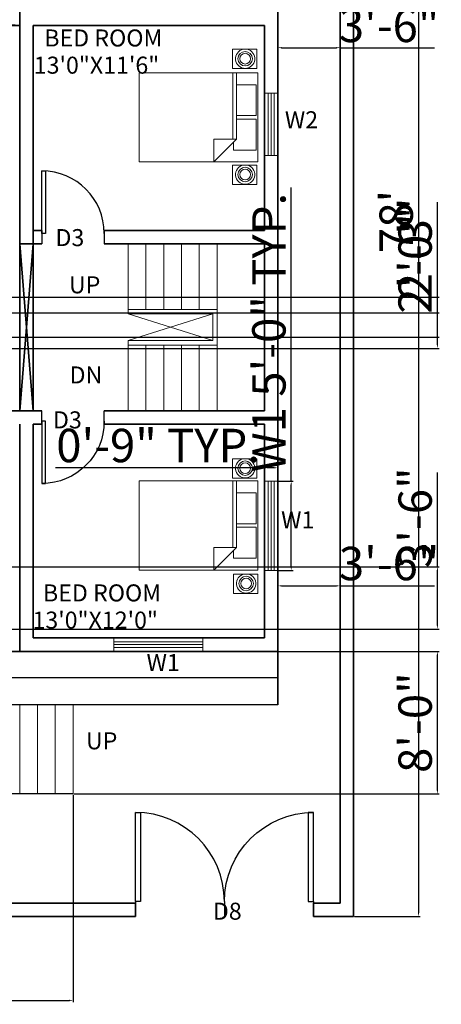
# Model space of a CAD drawing. Units: inches. Extents: x 164 to 1038, y 98 to 1358.
# Tile 3 of 4: x 754 to 1038, y 151 to 814. Entities that reach past the tile are written whole.
import ezdxf

# ---------------------------------------------------------------- set-up
doc = ezdxf.new("R2010")
doc.units = ezdxf.units.IN
for name, color, linetype, lineweight in [('A-ANNO-DIMS', 7, 'Continuous', 18), ('A-ANNO-TEXT', 3, 'Continuous', 18), ('A-AREA-IDEN', 3, 'Continuous', 18), ('A-FLOR', 7, 'Continuous', 25), ('C-SITE-GATE', 6, 'Continuous', 25), ('C-SITE-WALL', 7, 'Continuous', 35), ('door', 6, 'Continuous', 25), ('furniture', 2, 'Continuous', 18), ('staircase', 4, 'Continuous', 18), ('wall', 7, 'Continuous', 35), ('window', 10, 'Continuous', 18)]:
    doc.layers.add(name, color=color, linetype=linetype, lineweight=lineweight)
doc.styles.get("Standard").update_dxf_attribs({"font": 'arial.ttf'})
doc.dimstyles.new('ISO-25', dxfattribs={"dimtxt": 22.5, "dimasz": 2.5, "dimexe": 1.25, "dimexo": 0.625, "dimtad": 1, "dimdec": 0, "dimlunit": 3, "dimtxsty": 'Standard', "dimcen": 2.5, "dimadec": 0, "dimazin": 0, "dimtfac": 1, "dimtdec": 0, "dimtmove": 0, "dimatfit": 3, "dimfxl": 1, "dimarcsym": 0})

# ---------------------------------------------------------------- blocks, each defined once
blk = doc.blocks.new('*U3')
for p, q in [((0, 0), (0, -5)), ((30, 0), (30, -5))]:
    blk.add_line(p, q)
blk.add_lwpolyline([(0, 0), (0, 30), (1.75, 30), (1.75, 0)], close=True)
blk.add_arc((0, 0), 30, 0, 90)
blk = doc.blocks.new('Bed - Queen')
for p, q in [((0, -80.00003), (0, 0)), ((0, 0), (59.99999, 0)), ((59.99999, 0), (59.99999, -80.00003)), ((7.99999, -1.2), (28.79998, -1.2)), ((7.99999, -14.4), (7.99999, -1.2)), ((28.79998, -1.2), (28.79998, -14.4)), ((31.19999, -1.2), (51.99999, -1.2)), ((31.19999, -14.4), (31.19999, -1.2)), ((51.99999, -1.2), (51.99999, -16.4)), ((0, -14.4), (44.8, -14.4)), ((44.8, -16.8), (0, -16.8)), ((59.99999, -29.6), (44.8, -14.4)), ((44.8, -14.4), (44.8, -29.6)), ((51.99999, -16.4), (46.79936, -16.4)), ((44.8, -29.6), (59.99999, -29.6)), ((59.99999, -80.00003), (0, -80.00003))]:
    blk.add_line(p, q)
blk = doc.blocks.new('*D19')
at = {"layer": 'A-ANNO-DIMS', "color": 0, "lineweight": -2, "transparency": 16777216}
for p, q in [((979.69, 1145.87), (1024.11, 1145.87)), ((1022.86, 1143.37), (1022.86, 212.37)), ((979.69, 209.87), (1024.11, 209.87))]:
    blk.add_line(p, q, dxfattribs=at)
at = {"layer": 'A-ANNO-DIMS', "color": 0, "transparency": 16777216}
for points in [[(1022.44, 1143.37), (1023.28, 1143.37), (1022.86, 1145.87)], [(1022.44, 212.37), (1023.28, 212.37), (1022.86, 209.87)]]:
    blk.add_solid(points, dxfattribs=at)
at = {"layer": 'Defpoints', "color": 0, "transparency": 16777216}
for p in [(979.07, 1145.87), (979.07, 209.87), (1022.86, 209.87)]:
    blk.add_point(p, dxfattribs=at)
at = {"layer": 'A-ANNO-DIMS', "color": 0, "transparency": 16777216, "insert": (1010.75, 677.87), "char_height": 22.5, "attachment_point": 5, "rotation": 90}
blk.add_mtext("78'", dxfattribs=at)
blk = doc.blocks.new('*D25')
at = {"layer": 'A-ANNO-DIMS', "color": 0, "lineweight": -2, "transparency": 16777216}
for p, q in [((928.07, 429.88), (928.07, 433.73)), ((930.57, 432.48), (967.57, 432.48)), ((970.07, 429.88), (970.07, 433.73)), ((970.07, 432.48), (1033.61, 432.48))]:
    blk.add_line(p, q, dxfattribs=at)
at = {"layer": 'A-ANNO-DIMS', "color": 0, "transparency": 16777216}
for points in [[(930.57, 432.9), (930.57, 432.07), (928.07, 432.48)], [(967.57, 432.9), (967.57, 432.07), (970.07, 432.48)]]:
    blk.add_solid(points, dxfattribs=at)
at = {"layer": 'Defpoints', "color": 0, "transparency": 16777216}
for p in [(970.07, 432.48), (928.07, 429.26), (970.07, 429.26)]:
    blk.add_point(p, dxfattribs=at)
at = {"layer": 'A-ANNO-DIMS', "color": 0, "transparency": 16777216, "insert": (1003.09, 444.6), "char_height": 22.5, "attachment_point": 5}
blk.add_mtext('3\'-6"', dxfattribs=at)
blk = doc.blocks.new('*D28')
at = {"layer": 'A-ANNO-DIMS', "color": 0, "lineweight": -2, "transparency": 16777216}
for p, q in [((928.07, 772.18), (928.07, 796.13)), ((970.07, 772.18), (970.07, 796.13)), ((930.57, 794.88), (967.57, 794.88)), ((970.07, 794.88), (1033.61, 794.88))]:
    blk.add_line(p, q, dxfattribs=at)
at = {"layer": 'A-ANNO-DIMS', "color": 0, "transparency": 16777216}
for points in [[(930.57, 795.3), (930.57, 794.46), (928.07, 794.88)], [(967.57, 795.3), (967.57, 794.46), (970.07, 794.88)]]:
    blk.add_solid(points, dxfattribs=at)
at = {"layer": 'Defpoints', "color": 0, "transparency": 16777216}
for p in [(970.07, 794.88), (928.07, 771.56), (970.07, 771.56)]:
    blk.add_point(p, dxfattribs=at)
at = {"layer": 'A-ANNO-DIMS', "color": 0, "transparency": 16777216, "insert": (1003.09, 807), "char_height": 22.5, "attachment_point": 5}
blk.add_mtext('3\'-6"', dxfattribs=at)
blk = doc.blocks.new('WINDOW-W1')
for p, q in [((0, 9), (0, 0)), ((60.11, 9), (60.11, 0)), ((0, 6.5), (60.11, 6.5)), ((0, 4.5), (60.11, 4.5)), ((0, 2.5), (60.11, 2.5))]:
    blk.add_line(p, q)
blk = doc.blocks.new('WINDOW-W2')
for p, q in [((0, 9), (0, 0)), ((42.02, 9), (42.02, 0)), ((0, 6.5), (42.02, 6.5)), ((0, 4.5), (42.02, 4.5)), ((0, 2.5), (42.02, 2.5))]:
    blk.add_line(p, q)
blk = doc.blocks.new('BEDSIDE-TABLE')
blk.add_lwpolyline([(0, 13.01), (16.36, 13.01), (16.36, 0), (0, 0)], close=True)
for radius in [4.87, 3.63]:
    blk.add_circle((8.46, 6.65), radius)
blk.add_arc((8.46, 6.65), 6.51, 102.02927, 77.97073)
blk.add_arc((8.46, 6.65), 6.51, 102.02927, 77.97073)
blk = doc.blocks.new('*D34')
at = {"layer": 'A-ANNO-DIMS', "color": 0, "lineweight": -2, "transparency": 16777216}
for p, q in [((937.08, 502.97), (937.08, 700.67)), ((928.69, 502.97), (938.33, 502.97)), ((937.08, 445.36), (937.08, 500.47)), ((928.69, 442.86), (938.33, 442.86))]:
    blk.add_line(p, q, dxfattribs=at)
at = {"layer": 'A-ANNO-DIMS', "color": 0, "transparency": 16777216}
for points in [[(936.67, 500.47), (937.5, 500.47), (937.08, 502.97)], [(936.67, 445.36), (937.5, 445.36), (937.08, 442.86)]]:
    blk.add_solid(points, dxfattribs=at)
at = {"layer": 'Defpoints', "color": 0, "transparency": 16777216}
for p in [(928.07, 502.97), (937.08, 502.97), (928.07, 442.86)]:
    blk.add_point(p, dxfattribs=at)
at = {"layer": 'A-ANNO-DIMS', "color": 0, "transparency": 16777216, "insert": (924.97, 603.07), "char_height": 22.5, "attachment_point": 5, "rotation": 90}
blk.add_mtext('W1 5\'-0" TYP.', dxfattribs=at)
blk = doc.blocks.new('*D35')
at = {"layer": 'A-ANNO-DIMS', "color": 0, "lineweight": -2, "transparency": 16777216}
for p, q in [((919.07, 511.99), (778.17, 511.99)), ((919.07, 503.6), (919.07, 513.24)), ((925.57, 511.99), (921.57, 511.99)), ((928.07, 503.6), (928.07, 513.24))]:
    blk.add_line(p, q, dxfattribs=at)
at = {"layer": 'A-ANNO-DIMS', "color": 0, "transparency": 16777216}
for points in [[(921.57, 512.4), (921.57, 511.57), (919.07, 511.99)], [(925.57, 512.4), (925.57, 511.57), (928.07, 511.99)]]:
    blk.add_solid(points, dxfattribs=at)
at = {"layer": 'Defpoints', "color": 0, "transparency": 16777216}
for p in [(919.07, 511.99), (919.07, 502.97), (928.07, 502.97)]:
    blk.add_point(p, dxfattribs=at)
at = {"layer": 'A-ANNO-DIMS', "color": 0, "transparency": 16777216, "insert": (847.37, 524.1), "char_height": 22.5, "attachment_point": 5}
blk.add_mtext('0\'-9" TYP.', dxfattribs=at)
blk = doc.blocks.new('*D56')
at = {"layer": 'A-ANNO-DIMS', "color": 0, "lineweight": -2, "transparency": 16777216}
for p, q in [((1035.62, 616.37), (1035.62, 680.31)), ((510.19, 616.37), (1036.87, 616.37)), ((1035.62, 594.87), (1035.62, 613.87)), ((510.19, 592.37), (1036.87, 592.37))]:
    blk.add_line(p, q, dxfattribs=at)
at = {"layer": 'A-ANNO-DIMS', "color": 0, "transparency": 16777216}
for points in [[(1035.2, 613.87), (1036.03, 613.87), (1035.62, 616.37)], [(1035.2, 594.87), (1036.03, 594.87), (1035.62, 592.37)]]:
    blk.add_solid(points, dxfattribs=at)
at = {"layer": 'Defpoints', "color": 0, "transparency": 16777216}
for p in [(509.57, 616.37), (1035.62, 616.37), (509.57, 592.37)]:
    blk.add_point(p, dxfattribs=at)
at = {"layer": 'A-ANNO-DIMS', "color": 0, "transparency": 16777216, "insert": (1023.5, 649.59), "char_height": 22.5, "attachment_point": 5, "rotation": 90}
blk.add_mtext('2\'-0"', dxfattribs=at)
blk = doc.blocks.new('*D58')
at = {"layer": 'A-ANNO-DIMS', "color": 0, "lineweight": -2, "transparency": 16777216}
for p, q in [((1035.62, 626.87), (1035.62, 690.81)), ((400.69, 626.87), (1036.87, 626.87)), ((1035.62, 602.37), (1035.62, 624.37)), ((400.69, 599.87), (1036.87, 599.87))]:
    blk.add_line(p, q, dxfattribs=at)
at = {"layer": 'A-ANNO-DIMS', "color": 0, "transparency": 16777216}
for points in [[(1035.2, 624.37), (1036.03, 624.37), (1035.62, 626.87)], [(1035.2, 602.37), (1036.03, 602.37), (1035.62, 599.87)]]:
    blk.add_solid(points, dxfattribs=at)
at = {"layer": 'Defpoints', "color": 0, "transparency": 16777216}
for p in [(400.07, 626.87), (1035.62, 626.87), (400.07, 599.87)]:
    blk.add_point(p, dxfattribs=at)
at = {"layer": 'A-ANNO-DIMS', "color": 0, "transparency": 16777216, "insert": (1023.5, 660.09), "char_height": 22.5, "attachment_point": 5, "rotation": 90}
blk.add_mtext('2\'-3"', dxfattribs=at)
blk = doc.blocks.new('*D59')
at = {"layer": 'A-ANNO-DIMS', "color": 0, "lineweight": -2, "transparency": 16777216}
for p, q in [((1035.62, 445.37), (1035.62, 508.91)), ((607.69, 445.37), (1036.87, 445.37)), ((1035.62, 405.87), (1035.62, 442.87)), ((607.69, 403.37), (1036.87, 403.37))]:
    blk.add_line(p, q, dxfattribs=at)
at = {"layer": 'A-ANNO-DIMS', "color": 0, "transparency": 16777216}
for points in [[(1035.2, 442.87), (1036.03, 442.87), (1035.62, 445.37)], [(1035.2, 405.87), (1036.03, 405.87), (1035.62, 403.37)]]:
    blk.add_solid(points, dxfattribs=at)
at = {"layer": 'Defpoints', "color": 0, "transparency": 16777216}
for p in [(607.07, 445.37), (1035.62, 445.37), (607.07, 403.37)]:
    blk.add_point(p, dxfattribs=at)
at = {"layer": 'A-ANNO-DIMS', "color": 0, "transparency": 16777216, "insert": (1023.5, 478.39), "char_height": 22.5, "attachment_point": 5, "rotation": 90}
blk.add_mtext('3\'-6"', dxfattribs=at)
blk = doc.blocks.new('*D60')
at = {"layer": 'A-ANNO-DIMS', "color": 0, "lineweight": -2, "transparency": 16777216}
for p, q in [((568.07, 291.74), (568.07, 152.07)), ((790.07, 291.74), (790.07, 152.07)), ((570.57, 153.32), (787.57, 153.32))]:
    blk.add_line(p, q, dxfattribs=at)
at = {"layer": 'A-ANNO-DIMS', "color": 0, "transparency": 16777216}
for points in [[(570.57, 153.73), (570.57, 152.9), (568.07, 153.32)], [(787.57, 153.73), (787.57, 152.9), (790.07, 153.32)]]:
    blk.add_solid(points, dxfattribs=at)
at = {"layer": 'Defpoints', "color": 0, "transparency": 16777216}
for p in [(568.07, 292.37), (790.07, 292.37), (790.07, 153.32)]:
    blk.add_point(p, dxfattribs=at)
at = {"layer": 'A-ANNO-DIMS', "color": 0, "transparency": 16777216, "insert": (679.07, 165.43), "char_height": 22.5, "attachment_point": 5}
blk.add_mtext('18\'-6"', dxfattribs=at)
blk = doc.blocks.new('*D61')
at = {"layer": 'A-ANNO-DIMS', "color": 0, "lineweight": -2, "transparency": 16777216}
for p, q in [((928.69, 388.37), (1036.87, 388.37)), ((1035.62, 294.87), (1035.62, 385.87)), ((790.69, 292.37), (1036.87, 292.37))]:
    blk.add_line(p, q, dxfattribs=at)
at = {"layer": 'A-ANNO-DIMS', "color": 0, "transparency": 16777216}
for points in [[(1035.2, 385.87), (1036.03, 385.87), (1035.62, 388.37)], [(1035.2, 294.87), (1036.03, 294.87), (1035.62, 292.37)]]:
    blk.add_solid(points, dxfattribs=at)
at = {"layer": 'Defpoints', "color": 0, "transparency": 16777216}
for p in [(928.07, 388.37), (1035.62, 388.37), (790.07, 292.37)]:
    blk.add_point(p, dxfattribs=at)
at = {"layer": 'A-ANNO-DIMS', "color": 0, "transparency": 16777216, "insert": (1023.5, 340.37), "char_height": 22.5, "attachment_point": 5, "rotation": 90}
blk.add_mtext('8\'-0"', dxfattribs=at)

msp = doc.modelspace()

# ---------------------------------------------------------------- linework, layer by layer
at = {"layer": 'A-FLOR'}
for p, q in [((715.07, 370.73), (928.07, 370.73)), ((928.07, 370.73), (928.07, 370.73)), ((928.07, 352.37), (715.07, 352.37)), ((790.07, 292.37), (568.07, 292.37))]:
    msp.add_line(p, q, dxfattribs=at)
at = {"layer": 'C-SITE-WALL'}
for p, q in [((979.07, 1145.87), (979.07, 209.87)), ((970.07, 818.87), (970.07, 218.87)), ((832.07, 218.87), (487.07, 218.87)), ((832.07, 218.87), (832.07, 209.87)), ((970.07, 218.87), (952.07, 218.87)), ((952.07, 218.87), (952.07, 209.87)), ((832.07, 209.87), (487.07, 209.87)), ((979.07, 209.87), (952.07, 209.87))]:
    msp.add_line(p, q, dxfattribs=at)
at = {"layer": 'door'}
for p, q in [((769.07, 671.87), (769.07, 662.87)), ((811.07, 671.87), (811.07, 662.87)), ((769.07, 541.37), (769.07, 550.37)), ((811.07, 541.37), (811.07, 550.37))]:
    msp.add_line(p, q, dxfattribs=at)
at = {"layer": 'staircase'}
for p, q in [((827.15, 662.87), (827.15, 615.62)), ((839.15, 662.87), (839.15, 618.62)), ((851.15, 662.87), (851.15, 618.62)), ((863.15, 662.87), (863.15, 618.62)), ((875.15, 662.87), (875.15, 618.62)), ((887.15, 662.87), (887.15, 550.37)), ((887.15, 618.62), (827.15, 618.62)), ((884.15, 615.62), (827.15, 615.62)), ((827.15, 615.62), (884.15, 597.62)), ((884.15, 615.62), (827.15, 597.62)), ((884.15, 615.62), (884.15, 597.62)), ((884.15, 597.62), (827.15, 597.62)), ((827.15, 597.62), (827.15, 550.37)), ((887.15, 594.62), (827.15, 594.62)), ((839.15, 594.62), (839.15, 550.37)), ((851.15, 594.62), (851.15, 550.37)), ((863.15, 594.62), (863.15, 550.37)), ((875.15, 594.62), (875.15, 550.37)), ((754.07, 352.37), (754.07, 292.37)), ((766.07, 352.37), (766.07, 292.37)), ((778.07, 352.37), (778.07, 292.37)), ((790.07, 352.37), (790.07, 292.37))]:
    msp.add_line(p, q, dxfattribs=at)
at = {"layer": 'wall'}
for p, q in [((616.07, 818.87), (754.07, 809.87)), ((754.07, 818.87), (754.07, 550.37)), ((928.07, 818.87), (928.07, 352.37)), ((754.07, 809.87), (565.07, 809.87)), ((919.07, 809.87), (763.07, 809.87)), ((763.07, 809.87), (763.07, 550.37)), ((919.07, 809.87), (919.07, 671.87)), ((769.07, 671.87), (763.07, 671.87)), ((919.07, 671.87), (811.07, 671.87)), ((769.07, 662.87), (754.07, 662.87)), ((763.07, 662.87), (754.07, 550.37)), ((763.07, 550.37), (754.07, 662.87)), ((919.07, 662.87), (811.07, 662.87)), ((919.07, 662.87), (919.07, 550.37)), ((769.07, 550.37), (565.07, 550.37)), ((919.07, 550.37), (811.07, 550.37)), ((754.07, 541.37), (754.07, 388.37)), ((763.07, 541.37), (763.07, 397.37)), ((769.07, 541.37), (763.07, 541.37)), ((919.07, 541.37), (811.07, 541.37)), ((919.07, 541.37), (919.07, 397.37)), ((919.07, 397.37), (763.07, 397.37)), ((928.07, 388.37), (715.07, 388.37))]:
    msp.add_line(p, q, dxfattribs=at)

# ---------------------------------------------------------------- block references
at = {"layer": 'C-SITE-GATE', "yscale": 2, "zscale": 2}
for p, xscale in [((832.07, 219.87), 2), ((952.07, 219.87), -2)]:
    msp.add_blockref('*U3', p, dxfattribs=dict(at, xscale=xscale))
at = {"layer": 'door', "xscale": 1.400000000000005, "yscale": 1.400000000000005, "zscale": 1.400000000000005}
msp.add_blockref('*U3', (769.07, 669.87), dxfattribs=at)
at = {"layer": 'door', "xscale": -1.400000000000005, "yscale": 1.400000000000005, "zscale": 1.400000000000005, "rotation": 180}
msp.add_blockref('*U3', (769.07, 543.37), dxfattribs=at)
at = {"layer": 'furniture'}
for p in [(897.6, 780.84), (897.6, 702.83), (897.6, 505.06), (898.25, 427.41)]:
    msp.add_blockref('BEDSIDE-TABLE', p, dxfattribs=at)
at = {"layer": 'furniture', "rotation": 270}
for p in [(914.61, 777.99), (914.61, 503.13)]:
    msp.add_blockref('Bed - Queen', p, dxfattribs=at)
at = {"layer": 'window'}
for name, p, rotation in [('WINDOW-W2', (919.07, 764.24), 270.0000000000007), ('WINDOW-W1', (928.07, 442.86), 90.00000000000003), ('WINDOW-W1', (877.61, 397.37), 180)]:
    msp.add_blockref(name, p, dxfattribs=dict(at, rotation=rotation))

# ---------------------------------------------------------------- texts
at = {"layer": 'A-ANNO-TEXT'}
for s, p in [('W2', (932.8, 740.62)), ('D3', (778.18, 661.26)), ('UP', (787.26, 629.47)), ('DN', (787.71, 568.77)), ('D3', (776.5, 538.52)), ('W1', (930.27, 471.21)), ('W1', (839.58, 375.09)), ('UP', (798.74, 322.37)), ('D8', (884.28, 207.63))]:
    msp.add_text(s, height=11.466, dxfattribs=at).set_placement(p)
at = {"layer": 'A-AREA-IDEN'}
for s, height, p in [('BED ROOM', 11.466, (770.64, 795.71)), ('13\'0"X11\'6"', 11.4664, (763.56, 777.39)), ('BED ROOM', 11.466, (769.77, 421.98)), ('13\'0"X12\'0"', 11.4664, (762.69, 403.67))]:
    msp.add_text(s, height=height, dxfattribs=at).set_placement(p)

# ---------------------------------------------------------------- dimensions: what is measured, and where the dimension line sits
at = {"layer": 'A-ANNO-DIMS'}
for base, p1, p2, override, picture, middle in [((1022.86, 209.87), (979.07, 1145.87), (979.07, 209.87), {"dimclrd": 0, "dimclre": 0, "dimclrt": 0}, '*D19', (1010.75, 677.87)), ((1035.62, 626.87), (400.07, 599.87), (400.07, 626.87), {"dimdec": 1, "dimlfac": 1, "dimrnd": 0, "dimzin": 1, "dimdsep": 46, "dimlunit": 4, "dimfrac": 2}, '*D58', (1023.5, 660.09)), ((1035.62, 616.37), (509.57, 592.37), (509.57, 616.37), {"dimdec": 1, "dimlfac": 1, "dimrnd": 0, "dimzin": 1, "dimdsep": 46, "dimlunit": 4, "dimfrac": 2}, '*D56', (1023.5, 649.59)), ((1035.62, 445.37), (607.07, 403.37), (607.07, 445.37), {"dimdec": 1, "dimlfac": 1, "dimrnd": 0, "dimzin": 1, "dimdsep": 46, "dimlunit": 4, "dimfrac": 2}, '*D59', (1023.5, 478.39)), ((1035.62, 388.37), (790.07, 292.37), (928.07, 388.37), {"dimdec": 1, "dimlfac": 1, "dimrnd": 0, "dimzin": 1, "dimdsep": 46, "dimlunit": 4, "dimfrac": 2}, '*D61', (1023.5, 340.37))]:
    dim = msp.add_linear_dim(base=base, p1=p1, p2=p2, angle=90, dimstyle='ISO-25', override=override, dxfattribs=at)
    dim.commit()
    dim.dimension.update_dxf_attribs({"geometry": picture, "text_midpoint": middle})
for base, p1, p2, override, picture, middle in [((970.07, 794.88), (928.07, 771.56), (970.07, 771.56), {"dimclrd": 0, "dimclre": 0, "dimclrt": 0}, '*D28', (1003.09, 807)), ((970.07, 432.48), (928.07, 429.26), (970.07, 429.26), {"dimclrd": 0, "dimclre": 0, "dimclrt": 0}, '*D25', (1003.09, 444.6)), ((790.07, 153.32), (568.07, 292.37), (790.07, 292.37), {"dimdec": 1, "dimlfac": 1, "dimrnd": 0, "dimzin": 1, "dimdsep": 46, "dimlunit": 4, "dimfrac": 2}, '*D60', (679.07, 165.43))]:
    dim = msp.add_linear_dim(base=base, p1=p1, p2=p2, dimstyle='ISO-25', override=override, dxfattribs=at)
    dim.commit()
    dim.dimension.update_dxf_attribs({"geometry": picture, "text_midpoint": middle})
for base, p1, p2, angle, text, picture, middle in [((937.08, 502.97), (928.07, 442.86), (928.07, 502.97), 90, 'W1 <> TYP.', '*D34', (924.97, 603.07)), ((919.07, 511.99), (928.07, 502.97), (919.07, 502.97), 180, '<> TYP.', '*D35', (847.37, 524.1))]:
    dim = msp.add_linear_dim(base=base, p1=p1, p2=p2, angle=angle, text=text, dimstyle='ISO-25', override={"dimdec": 1, "dimlfac": 1, "dimrnd": 0, "dimzin": 1, "dimdsep": 46, "dimlunit": 4, "dimfrac": 2}, dxfattribs=at)
    dim.commit()
    dim.dimension.update_dxf_attribs({"geometry": picture, "text_midpoint": middle})

doc.saveas('drawing.dxf')
